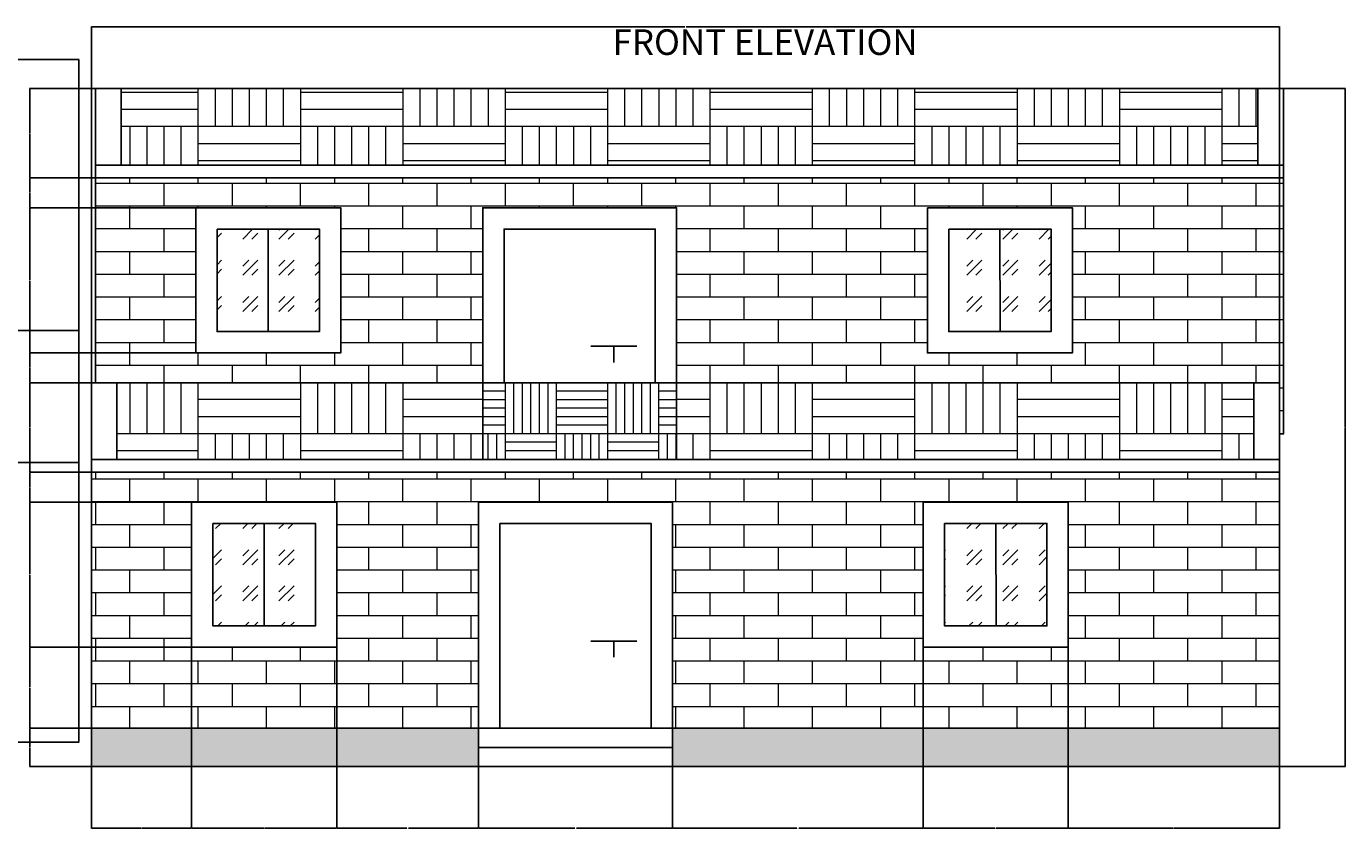
# Model space of a CAD drawing. Units: inches. Extents: x -73 to 1162, y -188 to 590.
# Tile 9 of 9: x 543 to 1162, y 199 to 575. Entities that reach past the tile are written whole.
import ezdxf

# ---------------------------------------------------------------- set-up
doc = ezdxf.new("R2010")
doc.units = ezdxf.units.IN
doc.header["$MEASUREMENT"] = 0
for name, color, linetype, lineweight in [('A-ANNO-DIMS', 2, 'Continuous', 18), ('A-ANNO-TEXT', 7, 'Continuous', 25), ('A-ELEV', 7, 'Continuous', 25), ('A-ELEV-PATT', 252, 'Continuous', 13)]:
    doc.layers.add(name, color=color, linetype=linetype, lineweight=lineweight)
doc.styles.get("Standard").update_dxf_attribs({"font": 'arial.ttf'})
doc.dimstyles.get("Standard").update_dxf_attribs({"dimtxt": 0.18, "dimasz": 0.18, "dimexe": 0.18, "dimexo": 0.0625, "dimgap": 0.09, "dimtad": 0, "dimtih": 1, "dimtoh": 1, "dimdec": 1, "dimzin": 0, "dimdsep": 46, "dimlunit": 4, "dimtxsty": 'Standard', "dimcen": 0.09, "dimadec": 0, "dimazin": 0, "dimtfac": 1, "dimtdec": 1, "dimtofl": 0, "dimtmove": 0, "dimatfit": 3, "dimfxl": 1, "dimtolj": 1, "dimtzin": 0, "dimarcsym": 0})

# ---------------------------------------------------------------- blocks, each defined once
blk = doc.blocks.new('*D141')
at = {"layer": 'A-ANNO-DIMS', "color": 0, "lineweight": -2, "transparency": 16777216}
for p, q in [((537.78, 559.33), (568.19, 559.33)), ((568.01, 559.15), (568.01, 399.52)), ((568.01, 239.52), (568.01, 399.15)), ((537.78, 239.34), (568.19, 239.34))]:
    blk.add_line(p, q, dxfattribs=at)
at = {"layer": 'A-ANNO-DIMS', "color": 0, "transparency": 16777216}
for points in [[(567.98, 559.15), (568.04, 559.15), (568.01, 559.33)], [(567.98, 239.52), (568.04, 239.52), (568.01, 239.34)]]:
    blk.add_solid(points, dxfattribs=at)
at = {"layer": 'Defpoints', "color": 0, "transparency": 16777216}
for p in [(537.71, 559.33), (568.01, 559.33), (537.71, 239.34)]:
    blk.add_point(p, dxfattribs=at)
at = {"layer": 'A-ANNO-DIMS', "color": 0, "transparency": 16777216, "insert": (568.01, 399.33), "char_height": 0.18, "attachment_point": 5}
blk.add_mtext('\\A1;320', dxfattribs=at)
blk = doc.blocks.new('*D142')
at = {"layer": 'A-ANNO-DIMS', "color": 0, "lineweight": -2, "transparency": 16777216}
for p, q in [((346.78, 432.33), (568.19, 432.33)), ((568.01, 432.15), (568.01, 401.51)), ((568.01, 370.51), (568.01, 401.15)), ((346.77, 370.33), (568.19, 370.33))]:
    blk.add_line(p, q, dxfattribs=at)
at = {"layer": 'A-ANNO-DIMS', "color": 0, "transparency": 16777216}
for points in [[(567.98, 432.15), (568.04, 432.15), (568.01, 432.33)], [(567.98, 370.51), (568.04, 370.51), (568.01, 370.33)]]:
    blk.add_solid(points, dxfattribs=at)
at = {"layer": 'Defpoints', "color": 0, "transparency": 16777216}
for p in [(346.71, 432.33), (568.01, 432.33), (346.71, 370.33)]:
    blk.add_point(p, dxfattribs=at)
at = {"layer": 'A-ANNO-DIMS', "color": 0, "transparency": 16777216, "insert": (568.01, 401.33), "char_height": 0.18, "attachment_point": 5}
blk.add_mtext('\\A1;62', dxfattribs=at)
blk = doc.blocks.new('*D143')
at = {"layer": 'A-ANNO-DIMS', "color": 0, "lineweight": -2, "transparency": 16777216}
for p, q in [((573.92, 227.88), (573.92, 574.9)), ((574.1, 574.72), (852.13, 574.72)), ((1130.74, 574.72), (852.71, 574.72)), ((1130.92, 227.88), (1130.92, 574.9))]:
    blk.add_line(p, q, dxfattribs=at)
at = {"layer": 'A-ANNO-DIMS', "color": 0, "transparency": 16777216}
for points in [[(574.1, 574.75), (574.1, 574.69), (573.92, 574.72)], [(1130.74, 574.75), (1130.74, 574.69), (1130.92, 574.72)]]:
    blk.add_solid(points, dxfattribs=at)
at = {"layer": 'Defpoints', "color": 0, "transparency": 16777216}
for p in [(1130.92, 574.72), (573.92, 227.82), (1130.92, 227.82)]:
    blk.add_point(p, dxfattribs=at)
at = {"layer": 'A-ANNO-DIMS', "color": 0, "transparency": 16777216, "insert": (852.42, 574.72), "char_height": 0.18, "attachment_point": 5}
blk.add_mtext('\\A1;557', dxfattribs=at)
blk = doc.blocks.new('*D144')
at = {"layer": 'A-ANNO-DIMS', "color": 0, "lineweight": -2, "transparency": 16777216}
for p, q in [((1132.91, 545.82), (1161.93, 545.82)), ((1161.75, 545.64), (1161.75, 387)), ((1161.75, 228), (1161.75, 386.64)), ((1130.98, 227.82), (1161.93, 227.82))]:
    blk.add_line(p, q, dxfattribs=at)
at = {"layer": 'A-ANNO-DIMS', "color": 0, "transparency": 16777216}
for points in [[(1161.72, 545.64), (1161.78, 545.64), (1161.75, 545.82)], [(1161.72, 228), (1161.78, 228), (1161.75, 227.82)]]:
    blk.add_solid(points, dxfattribs=at)
at = {"layer": 'Defpoints', "color": 0, "transparency": 16777216}
for p in [(1132.85, 545.82), (1130.92, 227.82), (1161.75, 227.82)]:
    blk.add_point(p, dxfattribs=at)
at = {"layer": 'A-ANNO-DIMS', "color": 0, "transparency": 16777216, "insert": (1161.75, 386.82), "char_height": 0.18, "attachment_point": 5}
blk.add_mtext('\\A1;318', dxfattribs=at)
blk = doc.blocks.new('*D145')
at = {"layer": 'A-ANNO-DIMS', "color": 0, "lineweight": -2, "transparency": 16777216}
for p, q in [((573.86, 245.82), (544.84, 245.82)), ((545.02, 245.64), (545.02, 237)), ((545.02, 228), (545.02, 236.64)), ((573.86, 227.82), (544.84, 227.82))]:
    blk.add_line(p, q, dxfattribs=at)
at = {"layer": 'A-ANNO-DIMS', "color": 0, "transparency": 16777216}
for points in [[(544.99, 245.64), (545.05, 245.64), (545.02, 245.82)], [(544.99, 228), (545.05, 228), (545.02, 227.82)]]:
    blk.add_solid(points, dxfattribs=at)
at = {"layer": 'Defpoints', "color": 0, "transparency": 16777216}
for p in [(545.02, 245.82), (573.92, 245.82), (573.92, 227.82)]:
    blk.add_point(p, dxfattribs=at)
at = {"layer": 'A-ANNO-DIMS', "color": 0, "transparency": 16777216, "insert": (545.02, 236.82), "char_height": 0.18, "attachment_point": 5}
blk.add_mtext('\\A1;18', dxfattribs=at)
blk = doc.blocks.new('*D146')
at = {"layer": 'A-ANNO-DIMS', "color": 0, "lineweight": -2, "transparency": 16777216}
for p, q in [((620.86, 283.82), (544.84, 283.82)), ((545.02, 283.64), (545.02, 265)), ((545.02, 246), (545.02, 264.64)), ((573.86, 245.82), (544.84, 245.82))]:
    blk.add_line(p, q, dxfattribs=at)
at = {"layer": 'A-ANNO-DIMS', "color": 0, "transparency": 16777216}
for points in [[(544.99, 283.64), (545.05, 283.64), (545.02, 283.82)], [(544.99, 246), (545.05, 246), (545.02, 245.82)]]:
    blk.add_solid(points, dxfattribs=at)
at = {"layer": 'Defpoints', "color": 0, "transparency": 16777216}
for p in [(545.02, 283.82), (620.92, 283.82), (573.92, 245.82)]:
    blk.add_point(p, dxfattribs=at)
at = {"layer": 'A-ANNO-DIMS', "color": 0, "transparency": 16777216, "insert": (545.02, 264.82), "char_height": 0.18, "attachment_point": 5}
blk.add_mtext('\\A1;38', dxfattribs=at)
blk = doc.blocks.new('*D147')
at = {"layer": 'A-ANNO-DIMS', "color": 0, "lineweight": -2, "transparency": 16777216}
for p, q in [((620.86, 351.82), (544.84, 351.82)), ((545.02, 351.64), (545.02, 318)), ((545.02, 284), (545.02, 317.64)), ((620.86, 283.82), (544.84, 283.82))]:
    blk.add_line(p, q, dxfattribs=at)
at = {"layer": 'A-ANNO-DIMS', "color": 0, "transparency": 16777216}
for points in [[(544.99, 351.64), (545.05, 351.64), (545.02, 351.82)], [(544.99, 284), (545.05, 284), (545.02, 283.82)]]:
    blk.add_solid(points, dxfattribs=at)
at = {"layer": 'Defpoints', "color": 0, "transparency": 16777216}
for p in [(545.02, 351.82), (620.92, 351.82), (620.92, 283.82)]:
    blk.add_point(p, dxfattribs=at)
at = {"layer": 'A-ANNO-DIMS', "color": 0, "transparency": 16777216, "insert": (545.02, 317.82), "char_height": 0.18, "attachment_point": 5}
blk.add_mtext('\\A1;68', dxfattribs=at)
blk = doc.blocks.new('*D148')
at = {"layer": 'A-ANNO-DIMS', "color": 0, "lineweight": -2, "transparency": 16777216}
for p, q in [((573.86, 365.82), (544.84, 365.82)), ((545.02, 365.64), (545.02, 359)), ((545.02, 352), (545.02, 358.64)), ((620.86, 351.82), (544.84, 351.82))]:
    blk.add_line(p, q, dxfattribs=at)
at = {"layer": 'A-ANNO-DIMS', "color": 0, "transparency": 16777216}
for points in [[(544.99, 365.64), (545.05, 365.64), (545.02, 365.82)], [(544.99, 352), (545.05, 352), (545.02, 351.82)]]:
    blk.add_solid(points, dxfattribs=at)
at = {"layer": 'Defpoints', "color": 0, "transparency": 16777216}
for p in [(545.02, 365.82), (573.92, 365.82), (620.92, 351.82)]:
    blk.add_point(p, dxfattribs=at)
at = {"layer": 'A-ANNO-DIMS', "color": 0, "transparency": 16777216, "insert": (545.02, 358.82), "char_height": 0.18, "attachment_point": 5}
blk.add_mtext('\\A1;14', dxfattribs=at)
blk = doc.blocks.new('*D149')
at = {"layer": 'A-ANNO-DIMS', "color": 0, "lineweight": -2, "transparency": 16777216}
for p, q in [((573.86, 407.82), (544.84, 407.82)), ((545.02, 407.64), (545.02, 387)), ((545.02, 366), (545.02, 386.64)), ((573.86, 365.82), (544.84, 365.82))]:
    blk.add_line(p, q, dxfattribs=at)
at = {"layer": 'A-ANNO-DIMS', "color": 0, "transparency": 16777216}
for points in [[(544.99, 407.64), (545.05, 407.64), (545.02, 407.82)], [(544.99, 366), (545.05, 366), (545.02, 365.82)]]:
    blk.add_solid(points, dxfattribs=at)
at = {"layer": 'Defpoints', "color": 0, "transparency": 16777216}
for p in [(545.02, 407.82), (573.92, 407.82), (573.92, 365.82)]:
    blk.add_point(p, dxfattribs=at)
at = {"layer": 'A-ANNO-DIMS', "color": 0, "transparency": 16777216, "insert": (545.02, 386.82), "char_height": 0.18, "attachment_point": 5}
blk.add_mtext('\\A1;42', dxfattribs=at)
blk = doc.blocks.new('*D150')
at = {"layer": 'A-ANNO-DIMS', "color": 0, "lineweight": -2, "transparency": 16777216}
for p, q in [((622.79, 421.82), (544.84, 421.82)), ((545.02, 421.64), (545.02, 415)), ((545.02, 408), (545.02, 414.64)), ((573.86, 407.82), (544.84, 407.82))]:
    blk.add_line(p, q, dxfattribs=at)
at = {"layer": 'A-ANNO-DIMS', "color": 0, "transparency": 16777216}
for points in [[(544.99, 421.64), (545.05, 421.64), (545.02, 421.82)], [(544.99, 408), (545.05, 408), (545.02, 407.82)]]:
    blk.add_solid(points, dxfattribs=at)
at = {"layer": 'Defpoints', "color": 0, "transparency": 16777216}
for p in [(545.02, 421.82), (622.85, 421.82), (573.92, 407.82)]:
    blk.add_point(p, dxfattribs=at)
at = {"layer": 'A-ANNO-DIMS', "color": 0, "transparency": 16777216, "insert": (545.02, 414.82), "char_height": 0.18, "attachment_point": 5}
blk.add_mtext('\\A1;14', dxfattribs=at)
blk = doc.blocks.new('*D151')
at = {"layer": 'A-ANNO-DIMS', "color": 0, "lineweight": -2, "transparency": 16777216}
for p, q in [((622.79, 489.82), (544.84, 489.82)), ((545.02, 489.64), (545.02, 456)), ((545.02, 422), (545.02, 455.64)), ((622.79, 421.82), (544.84, 421.82))]:
    blk.add_line(p, q, dxfattribs=at)
at = {"layer": 'A-ANNO-DIMS', "color": 0, "transparency": 16777216}
for points in [[(544.99, 489.64), (545.05, 489.64), (545.02, 489.82)], [(544.99, 422), (545.05, 422), (545.02, 421.82)]]:
    blk.add_solid(points, dxfattribs=at)
at = {"layer": 'Defpoints', "color": 0, "transparency": 16777216}
for p in [(545.02, 489.82), (622.85, 489.82), (622.85, 421.82)]:
    blk.add_point(p, dxfattribs=at)
at = {"layer": 'A-ANNO-DIMS', "color": 0, "transparency": 16777216, "insert": (545.02, 455.82), "char_height": 0.18, "attachment_point": 5}
blk.add_mtext('\\A1;68', dxfattribs=at)
blk = doc.blocks.new('*D152')
at = {"layer": 'A-ANNO-DIMS', "color": 0, "lineweight": -2, "transparency": 16777216}
for p, q in [((575.79, 503.82), (544.84, 503.82)), ((545.02, 503.64), (545.02, 497)), ((545.02, 490), (545.02, 496.64)), ((622.79, 489.82), (544.84, 489.82))]:
    blk.add_line(p, q, dxfattribs=at)
at = {"layer": 'A-ANNO-DIMS', "color": 0, "transparency": 16777216}
for points in [[(544.99, 503.64), (545.05, 503.64), (545.02, 503.82)], [(544.99, 490), (545.05, 490), (545.02, 489.82)]]:
    blk.add_solid(points, dxfattribs=at)
at = {"layer": 'Defpoints', "color": 0, "transparency": 16777216}
for p in [(545.02, 503.82), (575.85, 503.82), (622.85, 489.82)]:
    blk.add_point(p, dxfattribs=at)
at = {"layer": 'A-ANNO-DIMS', "color": 0, "transparency": 16777216, "insert": (545.02, 496.82), "char_height": 0.18, "attachment_point": 5}
blk.add_mtext('\\A1;14', dxfattribs=at)
blk = doc.blocks.new('*D153')
at = {"layer": 'A-ANNO-DIMS', "color": 0, "lineweight": -2, "transparency": 16777216}
for p, q in [((575.79, 545.82), (544.84, 545.82)), ((545.02, 545.64), (545.02, 525)), ((545.02, 504), (545.02, 524.64)), ((575.79, 503.82), (544.84, 503.82))]:
    blk.add_line(p, q, dxfattribs=at)
at = {"layer": 'A-ANNO-DIMS', "color": 0, "transparency": 16777216}
for points in [[(544.99, 545.64), (545.05, 545.64), (545.02, 545.82)], [(544.99, 504), (545.05, 504), (545.02, 503.82)]]:
    blk.add_solid(points, dxfattribs=at)
at = {"layer": 'Defpoints', "color": 0, "transparency": 16777216}
for p in [(545.02, 545.82), (575.85, 545.82), (575.85, 503.82)]:
    blk.add_point(p, dxfattribs=at)
at = {"layer": 'A-ANNO-DIMS', "color": 0, "transparency": 16777216, "insert": (545.02, 524.82), "char_height": 0.18, "attachment_point": 5}
blk.add_mtext('\\A1;42', dxfattribs=at)
blk = doc.blocks.new('*D154')
at = {"layer": 'A-ANNO-DIMS', "color": 0, "lineweight": -2, "transparency": 16777216}
for p, q in [((620.92, 283.76), (620.92, 198.74)), ((573.92, 227.76), (573.92, 198.74)), ((574.1, 198.92), (597.2, 198.92)), ((620.74, 198.92), (597.64, 198.92))]:
    blk.add_line(p, q, dxfattribs=at)
at = {"layer": 'A-ANNO-DIMS', "color": 0, "transparency": 16777216}
for points in [[(574.1, 198.95), (574.1, 198.89), (573.92, 198.92)], [(620.74, 198.95), (620.74, 198.89), (620.92, 198.92)]]:
    blk.add_solid(points, dxfattribs=at)
at = {"layer": 'Defpoints', "color": 0, "transparency": 16777216}
for p in [(620.92, 283.82), (573.92, 227.82), (620.92, 198.92)]:
    blk.add_point(p, dxfattribs=at)
at = {"layer": 'A-ANNO-DIMS', "color": 0, "transparency": 16777216, "insert": (597.42, 198.92), "char_height": 0.18, "attachment_point": 5}
blk.add_mtext('\\A1;47', dxfattribs=at)
blk = doc.blocks.new('*D155')
at = {"layer": 'A-ANNO-DIMS', "color": 0, "lineweight": -2, "transparency": 16777216}
for p, q in [((620.92, 283.76), (620.92, 198.74)), ((688.92, 283.76), (688.92, 198.74)), ((621.1, 198.92), (654.7, 198.92)), ((688.74, 198.92), (655.14, 198.92))]:
    blk.add_line(p, q, dxfattribs=at)
at = {"layer": 'A-ANNO-DIMS', "color": 0, "transparency": 16777216}
for points in [[(621.1, 198.95), (621.1, 198.89), (620.92, 198.92)], [(688.74, 198.95), (688.74, 198.89), (688.92, 198.92)]]:
    blk.add_solid(points, dxfattribs=at)
at = {"layer": 'Defpoints', "color": 0, "transparency": 16777216}
for p in [(620.92, 283.82), (688.92, 283.82), (688.92, 198.92)]:
    blk.add_point(p, dxfattribs=at)
at = {"layer": 'A-ANNO-DIMS', "color": 0, "transparency": 16777216, "insert": (654.92, 198.92), "char_height": 0.18, "attachment_point": 5}
blk.add_mtext('\\A1;68', dxfattribs=at)
blk = doc.blocks.new('*D156')
at = {"layer": 'A-ANNO-DIMS', "color": 0, "lineweight": -2, "transparency": 16777216}
for p, q in [((688.92, 283.76), (688.92, 198.74)), ((755.49, 227.76), (755.49, 198.74)), ((689.1, 198.92), (721.81, 198.92)), ((755.31, 198.92), (722.6, 198.92))]:
    blk.add_line(p, q, dxfattribs=at)
at = {"layer": 'A-ANNO-DIMS', "color": 0, "transparency": 16777216}
for points in [[(689.1, 198.95), (689.1, 198.89), (688.92, 198.92)], [(755.31, 198.95), (755.31, 198.89), (755.49, 198.92)]]:
    blk.add_solid(points, dxfattribs=at)
at = {"layer": 'Defpoints', "color": 0, "transparency": 16777216}
for p in [(688.92, 283.82), (755.49, 227.82), (755.49, 198.92)]:
    blk.add_point(p, dxfattribs=at)
at = {"layer": 'A-ANNO-DIMS', "color": 0, "transparency": 16777216, "insert": (722.21, 198.92), "char_height": 0.18, "attachment_point": 5}
blk.add_mtext('\\A1;66.57', dxfattribs=at)
blk = doc.blocks.new('*D157')
at = {"layer": 'A-ANNO-DIMS', "color": 0, "lineweight": -2, "transparency": 16777216}
for p, q in [((755.49, 227.76), (755.49, 198.74)), ((846.36, 227.76), (846.36, 198.74)), ((755.67, 198.92), (800.53, 198.92)), ((846.18, 198.92), (801.32, 198.92))]:
    blk.add_line(p, q, dxfattribs=at)
at = {"layer": 'A-ANNO-DIMS', "color": 0, "transparency": 16777216}
for points in [[(755.67, 198.95), (755.67, 198.89), (755.49, 198.92)], [(846.18, 198.95), (846.18, 198.89), (846.36, 198.92)]]:
    blk.add_solid(points, dxfattribs=at)
at = {"layer": 'Defpoints', "color": 0, "transparency": 16777216}
for p in [(755.49, 227.82), (846.36, 227.82), (846.36, 198.92)]:
    blk.add_point(p, dxfattribs=at)
at = {"layer": 'A-ANNO-DIMS', "color": 0, "transparency": 16777216, "insert": (800.92, 198.92), "char_height": 0.18, "attachment_point": 5}
blk.add_mtext('\\A1;90.87', dxfattribs=at)
blk = doc.blocks.new('*D158')
at = {"layer": 'A-ANNO-DIMS', "color": 0, "lineweight": -2, "transparency": 16777216}
for p, q in [((963.92, 283.76), (963.92, 198.74)), ((846.36, 227.76), (846.36, 198.74)), ((846.54, 198.92), (904.68, 198.92)), ((963.74, 198.92), (905.59, 198.92))]:
    blk.add_line(p, q, dxfattribs=at)
at = {"layer": 'A-ANNO-DIMS', "color": 0, "transparency": 16777216}
for points in [[(846.54, 198.95), (846.54, 198.89), (846.36, 198.92)], [(963.74, 198.95), (963.74, 198.89), (963.92, 198.92)]]:
    blk.add_solid(points, dxfattribs=at)
at = {"layer": 'Defpoints', "color": 0, "transparency": 16777216}
for p in [(963.92, 283.82), (846.36, 227.82), (963.92, 198.92)]:
    blk.add_point(p, dxfattribs=at)
at = {"layer": 'A-ANNO-DIMS', "color": 0, "transparency": 16777216, "insert": (905.14, 198.92), "char_height": 0.18, "attachment_point": 5}
blk.add_mtext('\\A1;117.57', dxfattribs=at)
blk = doc.blocks.new('*D159')
at = {"layer": 'A-ANNO-DIMS', "color": 0, "lineweight": -2, "transparency": 16777216}
for p, q in [((963.92, 283.76), (963.92, 198.74)), ((1031.92, 283.76), (1031.92, 198.74)), ((964.1, 198.92), (997.7, 198.92)), ((1031.74, 198.92), (998.14, 198.92))]:
    blk.add_line(p, q, dxfattribs=at)
at = {"layer": 'A-ANNO-DIMS', "color": 0, "transparency": 16777216}
for points in [[(964.1, 198.95), (964.1, 198.89), (963.92, 198.92)], [(1031.74, 198.95), (1031.74, 198.89), (1031.92, 198.92)]]:
    blk.add_solid(points, dxfattribs=at)
at = {"layer": 'Defpoints', "color": 0, "transparency": 16777216}
for p in [(963.92, 283.82), (1031.92, 283.82), (1031.92, 198.92)]:
    blk.add_point(p, dxfattribs=at)
at = {"layer": 'A-ANNO-DIMS', "color": 0, "transparency": 16777216, "insert": (997.92, 198.92), "char_height": 0.18, "attachment_point": 5}
blk.add_mtext('\\A1;68', dxfattribs=at)
blk = doc.blocks.new('*D160')
at = {"layer": 'A-ANNO-DIMS', "color": 0, "lineweight": -2, "transparency": 16777216}
for p, q in [((1031.92, 283.76), (1031.92, 198.74)), ((1130.92, 227.76), (1130.92, 198.74)), ((1032.1, 198.92), (1081.2, 198.92)), ((1130.74, 198.92), (1081.64, 198.92))]:
    blk.add_line(p, q, dxfattribs=at)
at = {"layer": 'A-ANNO-DIMS', "color": 0, "transparency": 16777216}
for points in [[(1032.1, 198.95), (1032.1, 198.89), (1031.92, 198.92)], [(1130.74, 198.95), (1130.74, 198.89), (1130.92, 198.92)]]:
    blk.add_solid(points, dxfattribs=at)
at = {"layer": 'Defpoints', "color": 0, "transparency": 16777216}
for p in [(1031.92, 283.82), (1130.92, 227.82), (1130.92, 198.92)]:
    blk.add_point(p, dxfattribs=at)
at = {"layer": 'A-ANNO-DIMS', "color": 0, "transparency": 16777216, "insert": (1081.42, 198.92), "char_height": 0.18, "attachment_point": 5}
blk.add_mtext('\\A1;99', dxfattribs=at)

msp = doc.modelspace()

# ---------------------------------------------------------------- hatches: boundary and pattern name
at = {"layer": 'A-ELEV-PATT'}
h = msp.add_hatch(dxfattribs=at)
h.set_pattern_fill('AR-PARQ1', color=256, scale=4)
h.paths.add_polyline_path([(1120.8507, 545.8186), (587.8507, 545.8186), (587.8507, 509.8186), (1120.8507, 509.8186)])
h.paths.add_polyline_path([(757.4176, 407.8186), (585.9221, 407.8186), (585.9221, 371.8186), (757.4176, 371.8186)])
h.paths.add_polyline_path([(1118.9221, 407.8186), (848.2837, 407.8186), (848.2837, 371.8186), (1118.9221, 371.8186)])
h = msp.add_hatch(dxfattribs=at)
h.set_pattern_fill('AR-BRSTD', color=256, scale=4)
h.paths.add_polyline_path([(755.489, 351.8186), (846.3551, 351.8186), (846.3551, 245.8186), (1130.9221, 245.8186), (1130.9221, 365.8186), (573.9221, 365.8186), (573.9221, 245.8186), (755.489, 245.8186)])
h.paths.add_polyline_path([(620.9221, 351.8186), (688.9221, 351.8186), (688.9221, 283.8186), (620.9221, 283.8186)], flags=16)
h.paths.add_polyline_path([(630.9221, 341.8186), (678.9221, 341.8186), (678.9221, 293.8186), (630.9221, 293.8186)], flags=0)
h.paths.add_polyline_path([(963.9221, 351.8186), (1031.9221, 351.8186), (1031.9221, 283.8186), (963.9221, 283.8186)], flags=16)
h.paths.add_polyline_path([(973.9221, 341.8186), (1021.9221, 341.8186), (1021.9221, 293.8186), (973.9221, 293.8186)], flags=0)
h.paths.add_polyline_path([(757.4176, 489.8186), (848.2837, 489.8186), (848.2837, 407.8186), (1130.9221, 407.8186), (1130.9221, 383.8186), (1132.8507, 383.8186), (1132.8507, 503.8186), (575.8507, 503.8186), (575.8507, 407.8186), (757.4176, 407.8186)])
h.paths.add_polyline_path([(622.8507, 489.8186), (690.8507, 489.8186), (690.8507, 421.8186), (622.8507, 421.8186)], flags=16)
h.paths.add_polyline_path([(632.8507, 479.8186), (680.8507, 479.8186), (680.8507, 431.8186), (632.8507, 431.8186)], flags=0)
h.paths.add_polyline_path([(965.8507, 489.8186), (1033.8507, 489.8186), (1033.8507, 421.8186), (965.8507, 421.8186)], flags=16)
h.paths.add_polyline_path([(975.8507, 479.8186), (1023.8507, 479.8186), (1023.8507, 431.8186), (975.8507, 431.8186)], flags=0)
h = msp.add_hatch(dxfattribs=at)
h.set_pattern_fill('GOST_GLASS', color=256, scale=2)
h.set_pattern_definition([(45, (0, 0), (16.97056, -2e-15), [10, -14]), (45, (4.243, 0), (16.97056, -2e-15), [4, -20]), (45, (0, 4.243), (16.97056, -2e-15), [4, -20])])
h.paths.add_polyline_path([(654.9221, 341.8186), (630.9221, 341.8186), (630.9221, 293.8186), (654.9221, 293.8186)])
h.paths.add_polyline_path([(678.9221, 341.8186), (654.9221, 341.8186), (654.9221, 293.8186), (678.9221, 293.8186)])
h.paths.add_polyline_path([(997.9221, 341.8186), (973.9221, 341.8186), (973.9221, 293.8186), (998.0625, 293.8186)])
h.paths.add_polyline_path([(1021.9221, 341.8186), (997.9221, 341.8186), (998.0625, 293.8186), (1021.9221, 293.8186)])
h.paths.add_polyline_path([(656.8507, 479.8186), (632.8507, 479.8186), (632.8507, 431.8186), (656.8507, 431.8186)])
h.paths.add_polyline_path([(680.8507, 479.8186), (656.8507, 479.8186), (656.8507, 431.8186), (680.8507, 431.8186)])
h.paths.add_polyline_path([(999.8507, 479.8186), (975.8507, 479.8186), (975.8507, 431.8186), (999.9911, 431.8186)])
h.paths.add_polyline_path([(1023.8507, 479.8186), (999.8507, 479.8186), (999.9911, 431.8186), (1023.8507, 431.8186)])
h = msp.add_hatch(dxfattribs=at)
h.set_pattern_fill('AR-PARQ1', color=256, scale=2)
h.paths.add_polyline_path([(848.2837, 407.8186), (757.4176, 407.8186), (757.4176, 371.8186), (848.2837, 371.8186)])
h = msp.add_hatch(dxfattribs=at)
h.set_pattern_fill('AR-CONC', color=256, scale=2)
h.set_pattern_definition([(50, (0, 0), (14.3452, -1.25504), [1.5, -16.5]), (355, (0, 0), (-2.77503, 15.04384), [1.2, -13.2]), (100.4514, (1.195, -0.105), (11.57018, 13.7888), [1.2748, -14.02284]), (46.1842, (0, 4), (21.34483, -3.31039), [2.25, -24.75]), (96.6356, (1.779, 3.724), (18.69324, 19.48237), [1.9122, -21.03428]), (351.1842, (0, 4), (18.69324, 19.48237), [1.8, -19.8]), (21, (2, 3), (11.93814, -8.05238), [1.5, -16.5]), (326, (2, 3), (4.8663, 14.503), [1.2, -13.2]), (71.4514, (2.995, 2.329), (16.80445, 6.45062), [1.2748, -14.02284]), (37.5, (0, 0), (0.243197, 6.657877), [0, -13.04, 0, -13.4, 0, -13.25]), (7.5, (0, 0), (5.26139, 7.888234), [0, -7.64, 0, -12.74, 0, -5.05]), (327.5, (-4.46, 0), (10.676449, -0.451097), [0, -5, 0, -15.6, 0, -20.7]), (317.5, (-6.46, 0), (11.66372, 2.0021), [0, -6.5, 0, -10.36, 0, -14.7])])
h.paths.add_polyline_path([(755.489, 245.8186), (573.9221, 245.8186), (573.9221, 227.8186), (755.489, 227.8186)])
h.paths.add_polyline_path([(1130.9221, 245.8186), (846.3551, 245.8186), (846.3551, 227.8186), (1130.9221, 227.8186)])

# ---------------------------------------------------------------- linework, layer by layer
at = {"layer": 'A-ELEV'}
for p, q in [((575.8507, 545.8186), (1132.8507, 545.8186)), ((587.8507, 545.8186), (587.8507, 509.8186)), ((1120.8507, 545.8186), (1120.8507, 509.8186)), ((575.8507, 509.8186), (1132.8507, 509.8186)), ((575.8507, 503.8186), (1132.8507, 503.8186)), ((656.8507, 479.8186), (656.8507, 431.8186)), ((999.8507, 479.8186), (999.9911, 431.8186)), ((808.0803, 424.9544), (829.5936, 424.9544)), ((818.837, 424.9544), (818.837, 417.3433)), ((573.9221, 407.8186), (1130.9221, 407.8186)), ((573.9221, 407.8186), (1130.9221, 407.8186)), ((585.9221, 407.8186), (585.9221, 371.8186)), ((1118.9221, 407.8186), (1118.9221, 371.8186)), ((848, 383.8186), (848.2837, 383.8186)), ((1130.9221, 383.8186), (1132.8507, 383.8186)), ((573.9221, 371.8186), (1130.9221, 371.8186)), ((848, 374.8186), (848.2837, 374.8186)), ((573.9221, 365.8186), (1130.9221, 365.8186)), ((654.9221, 341.8186), (654.9221, 293.8186)), ((997.9221, 341.8186), (998.0625, 293.8186)), ((808.0803, 286.7009), (829.5936, 286.7009)), ((818.837, 286.7009), (818.837, 279.0898)), ((573.9221, 245.8186), (1130.9221, 245.8186)), ((755.489, 245.8186), (846.3551, 245.8186)), ((755.489, 236.8186), (846.3551, 236.8186)), ((573.9221, 227.8186), (1130.9221, 227.8186))]:
    msp.add_line(p, q, dxfattribs=at)
for points in [[(575.8507, 545.8186), (1132.8507, 545.8186), (1132.8507, 509.8186), (575.8507, 509.8186)], [(575.8507, 509.8186), (1132.8507, 509.8186), (1132.8507, 503.8186), (575.8507, 503.8186)], [(622.8507, 489.8186), (690.8507, 489.8186), (690.8507, 421.8186), (622.8507, 421.8186)], [(965.8507, 489.8186), (1033.8507, 489.8186), (1033.8507, 421.8186), (965.8507, 421.8186)], [(632.8507, 479.8186), (680.8507, 479.8186), (680.8507, 431.8186), (632.8507, 431.8186)], [(975.8507, 479.8186), (1023.8507, 479.8186), (1023.8507, 431.8186), (975.8507, 431.8186)], [(573.9221, 407.8186), (1130.9221, 407.8186), (1130.9221, 371.8186), (573.9221, 371.8186)], [(573.9221, 371.8186), (1130.9221, 371.8186), (1130.9221, 365.8186), (573.9221, 365.8186)], [(573.9221, 365.8186), (1130.9221, 365.8186), (1130.9221, 245.8186), (573.9221, 245.8186)], [(620.9221, 351.8186), (688.9221, 351.8186), (688.9221, 283.8186), (620.9221, 283.8186)], [(963.9221, 351.8186), (1031.9221, 351.8186), (1031.9221, 283.8186), (963.9221, 283.8186)], [(630.9221, 341.8186), (678.9221, 341.8186), (678.9221, 293.8186), (630.9221, 293.8186)], [(765.489, 341.8186), (836.3551, 341.8186), (836.3551, 245.8186), (765.489, 245.8186)], [(973.9221, 341.8186), (1021.9221, 341.8186), (1021.9221, 293.8186), (973.9221, 293.8186)], [(573.9221, 245.8186), (1130.9221, 245.8186), (1130.9221, 227.8186), (573.9221, 227.8186)]]:
    msp.add_lwpolyline(points, close=True, dxfattribs=at)
for points in [[(575.8507, 407.8186), (575.8507, 503.8186), (1132.8507, 503.8186), (1132.8507, 383.8186), (1130.9221, 383.8186)], [(757.4176, 371.8186), (757.4176, 489.8186), (848.2837, 489.8186), (848.2837, 371.8186)], [(767.4176, 407.8186), (767.4176, 479.8186), (838.2837, 479.8186), (838.2837, 407.8186)], [(755.489, 227.8186), (755.489, 351.8186), (846.3551, 351.8186), (846.3551, 227.8186)]]:
    msp.add_lwpolyline(points, dxfattribs=at)

# ---------------------------------------------------------------- texts
at = {"layer": 'A-ANNO-TEXT', "insert": (818.2726, 573.5129), "char_height": 12, "attachment_point": 1}
msp.add_mtext_dynamic_manual_height_columns('FRONT ELEVATION', width=198.609453, gutter_width=1, heights=[0], dxfattribs=at)

# ---------------------------------------------------------------- dimensions: what is measured, and where the dimension line sits
at = {"layer": 'A-ANNO-DIMS'}
for base, p1, p2, override, picture, middle in [((1130.9221, 574.7186), (573.9221, 227.8186), (1130.9221, 227.8186), {"dimdec": 0, "dimlfac": 1, "dimrnd": 0, "dimzin": 0, "dimdsep": 46, "dimlunit": 2}, '*D143', (852.4221, 574.7186)), ((620.9221, 198.9186), (573.9221, 227.8186), (620.9221, 283.8186), {"dimdec": 0, "dimlfac": 1, "dimrnd": 0, "dimzin": 0, "dimdsep": 46, "dimlunit": 2}, '*D154', (597.4221, 198.9186)), ((688.9221, 198.9186), (620.9221, 283.8186), (688.9221, 283.8186), {"dimdec": 0, "dimlfac": 1, "dimrnd": 0, "dimzin": 0, "dimdsep": 46, "dimlunit": 2}, '*D155', (654.9221, 198.9186)), ((755.489, 198.9186), (688.9221, 283.8186), (755.489, 227.8186), {"dimdec": 2, "dimlfac": 1, "dimrnd": 0, "dimzin": 0, "dimdsep": 46, "dimlunit": 2}, '*D156', (722.2055, 198.9186)), ((963.9221, 198.9186), (846.3551, 227.8186), (963.9221, 283.8186), {"dimdec": 2, "dimlfac": 1, "dimrnd": 0, "dimzin": 0, "dimdsep": 46, "dimlunit": 2}, '*D158', (905.1386, 198.9186)), ((1031.9221, 198.9186), (963.9221, 283.8186), (1031.9221, 283.8186), {"dimdec": 0, "dimlfac": 1, "dimrnd": 0, "dimzin": 0, "dimdsep": 46, "dimlunit": 2}, '*D159', (997.9221, 198.9186)), ((1130.9221, 198.9186), (1031.9221, 283.8186), (1130.9221, 227.8186), {"dimdec": 0, "dimlfac": 1, "dimrnd": 0, "dimzin": 0, "dimdsep": 46, "dimlunit": 2}, '*D160', (1081.4221, 198.9186)), ((846.3551, 198.9186), (755.489, 227.8186), (846.3551, 227.8186), {"dimdec": 2, "dimlfac": 1, "dimrnd": 0, "dimzin": 0, "dimdsep": 46, "dimlunit": 2}, '*D157', (800.9221, 198.9186))]:
    dim = msp.add_linear_dim(base=base, p1=p1, p2=p2, dimstyle='Standard', override=override, dxfattribs=at)
    dim.commit()
    dim.dimension.update_dxf_attribs({"geometry": picture, "text_midpoint": middle})
for base, p1, p2, picture, middle in [((568.013, 559.3321), (537.713, 239.3368), (537.713, 559.3321), '*D141', (568.013, 399.3345)), ((545.0221, 545.8186), (575.8507, 503.8186), (575.8507, 545.8186), '*D153', (545.0221, 524.8186)), ((1161.7507, 227.8186), (1132.8507, 545.8186), (1130.9221, 227.8186), '*D144', (1161.7507, 386.8186)), ((545.0221, 503.8186), (622.8507, 489.8186), (575.8507, 503.8186), '*D152', (545.0221, 496.8186)), ((545.0221, 489.8186), (622.8507, 421.8186), (622.8507, 489.8186), '*D151', (545.0221, 455.8186)), ((568.013, 432.3321), (346.7103, 370.3313), (346.713, 432.3321), '*D142', (568.013, 401.3317)), ((545.0221, 421.8186), (573.9221, 407.8186), (622.8507, 421.8186), '*D150', (545.0221, 414.8186)), ((545.0221, 407.8186), (573.9221, 365.8186), (573.9221, 407.8186), '*D149', (545.0221, 386.8186)), ((545.0221, 365.8186), (620.9221, 351.8186), (573.9221, 365.8186), '*D148', (545.0221, 358.8186)), ((545.0221, 351.8186), (620.9221, 283.8186), (620.9221, 351.8186), '*D147', (545.0221, 317.8186)), ((545.0221, 283.8186), (573.9221, 245.8186), (620.9221, 283.8186), '*D146', (545.0221, 264.8186)), ((545.0221, 245.8186), (573.9221, 227.8186), (573.9221, 245.8186), '*D145', (545.0221, 236.8186))]:
    dim = msp.add_linear_dim(base=base, p1=p1, p2=p2, angle=90, dimstyle='Standard', override={"dimdec": 0, "dimlfac": 1, "dimrnd": 0, "dimzin": 0, "dimdsep": 46, "dimlunit": 2}, dxfattribs=at)
    dim.commit()
    dim.dimension.update_dxf_attribs({"geometry": picture, "text_midpoint": middle})

doc.saveas('drawing.dxf')
